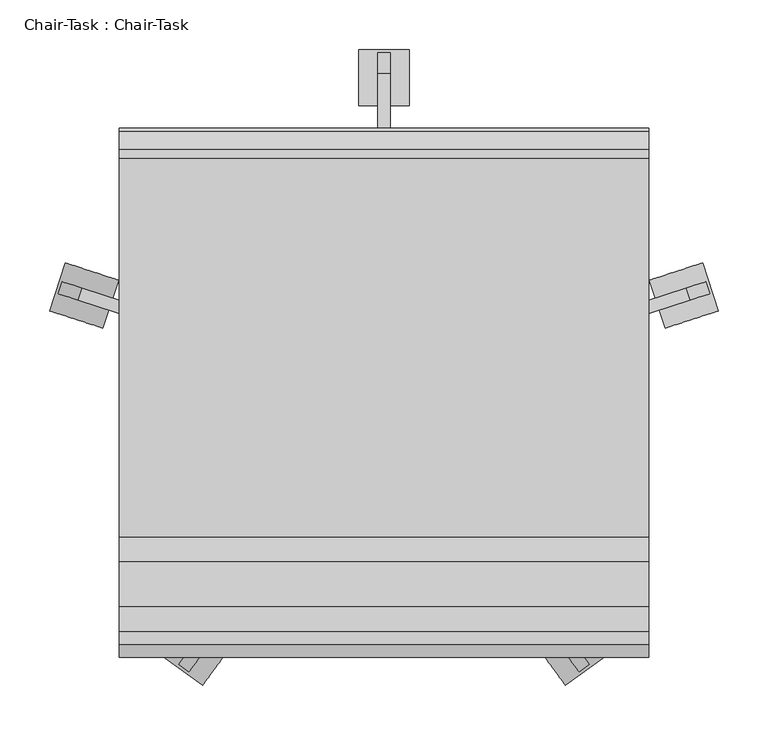
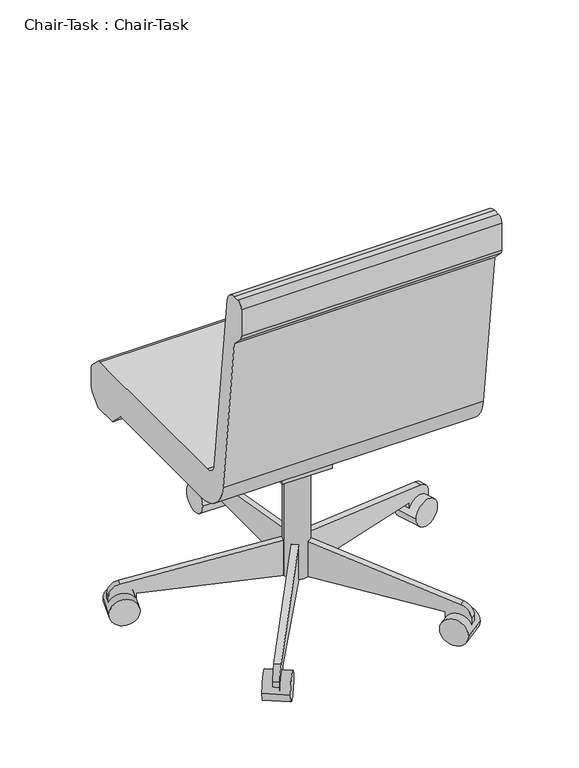
"""IFC4 building model written with IfcOpenShell, lengths in millimetres: furniture geometry, Chair-Task : Chair-Task."""

from ifc_helpers import new_model, si_unit, point, frame, frame_2d, origin, place, context, project, spatial, polyline, circle_curve, trimmed, segment, composite_curve, outline, extrude, source, transform, mapped, element, save


def chair_task_chair_task_b7f3823b(model_context):
    return source(origin(), model_context, "Body", "SweptSolid", [
        extrude(outline(composite_curve([segment(trimmed(circle_curve(frame_2d((140.9908197, 18.9459016)), 25.4), [point((115.5908197, 18.9459016))], [point((166.3908197, 18.9459016))], False, "CARTESIAN"), True, "CONTINUOUS"), segment(trimmed(circle_curve(frame_2d((140.9908197, 18.9459016)), 25.4), [point((166.3908197, 18.9459016))], [point((115.5908197, 18.9459016))], False, "CARTESIAN"), True, "CONTINUOUS")], self_intersect=False)), frame((0.0, 0.0, 53.5835944), z_axis=(0.0, 0.0, 1.0), x_axis=(1.0, 0.0, 0.0)), (0.0, 0.0, 1.0), 330.5914056),
        extrude(outline(composite_curve([segment(trimmed(circle_curve(frame_2d((0.0, -28.2002727)), 28.2002727), [point((0.0, -56.4005455))], [point((0.0, 0.0))], False, "CARTESIAN"), True, "CONTINUOUS"), segment(trimmed(circle_curve(frame_2d((0.0, -28.2002727)), 28.2002727), [point((0.0, 0.0))], [point((0.0, -56.4005455))], False, "CARTESIAN"), True, "CONTINUOUS")], self_intersect=False)), frame((477.6203484, 101.6163254, 28.1835944), z_axis=(-0.3090169943749423, 0.9510565162951553, 0.0), x_axis=(0.0, 0.0, 1.0)), (0.0, 0.0, 1.0), 50.8),
        extrude(outline(composite_curve([segment(polyline([(-25.4, 0.0), (0.0, 0.0), (0.0, -50.8), (-24.303053, -50.8)]), True, "CONTINUOUS"), segment(trimmed(circle_curve(frame_2d((-24.303053, -25.4)), 25.4), [point((-24.303053, -50.8))], [point((-49.3171699, -29.8106637))], False, "CARTESIAN"), True, "CONTINUOUS"), segment(polyline([(-49.3171699, -29.8106637), (-101.6, 266.7), (-101.6, 292.1), (-25.4, 292.1), (-25.4, 0.0)]), True, "CONTINUOUS")], self_intersect=False)), frame((420.756686, 103.1705568, 28.1835944), z_axis=(-0.3090169943749423, 0.9510565162951553, 0.0), x_axis=(0.0, 0.0, -1.0)), (0.0, 0.0, 1.0), 12.7),
        extrude(outline(composite_curve([segment(trimmed(circle_curve(frame_2d((0.0, -28.2002727)), 28.2002727), [point((0.0, -56.4005455))], [point((0.0, 0.0))], False, "CARTESIAN"), True, "CONTINUOUS"), segment(trimmed(circle_curve(frame_2d((0.0, -28.2002727)), 28.2002727), [point((0.0, 0.0))], [point((0.0, -56.4005455))], False, "CARTESIAN"), True, "CONTINUOUS")], self_intersect=False)), frame((323.63931, -275.6612394, 28.1835944), z_axis=(0.8090169943749499, 0.5877852522924699, 0.0), x_axis=(0.0, 0.0, 1.0)), (0.0, 0.0, 1.0), 50.8),
        extrude(outline(composite_curve([segment(polyline([(-25.4, 0.0), (0.0, 0.0), (0.0, -50.8), (-24.303053, -50.8)]), True, "CONTINUOUS"), segment(trimmed(circle_curve(frame_2d((-24.303053, -25.3999999)), 25.4), [point((-24.303053, -50.8))], [point((-49.3171699, -29.8106636))], False, "CARTESIAN"), True, "CONTINUOUS"), segment(polyline([(-49.3171699, -29.8106636), (-101.6, 266.7), (-101.6, 292.1), (-25.4, 292.1), (-25.4, 0.0)]), True, "CONTINUOUS")], self_intersect=False)), frame((307.545634, -221.1003988, 28.1835944), z_axis=(0.8090169943749499, 0.5877852522924699, 0.0), x_axis=(0.0, 0.0, -1.0)), (0.0, 0.0, 1.0), 12.7),
        extrude(outline(composite_curve([segment(trimmed(circle_curve(frame_2d((0.0, -28.2002727)), 28.2002727), [point((0.0, -56.4005455))], [point((0.0, 0.0))], False, "CARTESIAN"), True, "CONTINUOUS"), segment(trimmed(circle_curve(frame_2d((0.0, -28.2002727)), 28.2002727), [point((0.0, 0.0))], [point((0.0, -56.4005455))], False, "CARTESIAN"), True, "CONTINUOUS")], self_intersect=False)), frame((-41.6576707, -275.6612394, 28.1835944), z_axis=(-0.8090169943749458, 0.5877852522924754, 0.0), x_axis=(0.0, 0.0, -1.0)), (0.0, 0.0, 1.0), 50.8),
        extrude(outline(composite_curve([segment(polyline([(25.4, 0.0), (25.4, 292.1), (101.6, 292.1), (101.6, 266.7), (49.3171699, -29.8106637)]), True, "CONTINUOUS"), segment(trimmed(circle_curve(frame_2d((24.303053, -25.3999999)), 25.4), [point((49.3171699, -29.8106637))], [point((24.303053, -50.8))], False, "CARTESIAN"), True, "CONTINUOUS"), segment(polyline([(24.303053, -50.8), (0.0, -50.8), (0.0, 0.0), (25.4, 0.0)]), True, "CONTINUOUS")], self_intersect=False)), frame((-25.5639946, -221.1003988, 28.1835944), z_axis=(-0.8090169943749459, 0.5877852522924754, 0.0), x_axis=(0.0, 0.0, 1.0)), (0.0, 0.0, 1.0), 12.7),
        extrude(outline(composite_curve([segment(trimmed(circle_curve(frame_2d((0.0, -28.2002727)), 28.2002727), [point((0.0, -56.4005454))], [point((0.0, 0.0))], False, "CARTESIAN"), True, "CONTINUOUS"), segment(trimmed(circle_curve(frame_2d((0.0, -28.2002727)), 28.2002727), [point((0.0, 0.0))], [point((0.0, -56.4005454))], False, "CARTESIAN"), True, "CONTINUOUS")], self_intersect=False)), frame((-195.638709, 101.6163254, 28.1835944), z_axis=(0.3090169943749487, 0.9510565162951532, 0.0), x_axis=(0.0, 0.0, -1.0)), (0.0, 0.0, 1.0), 50.8),
        extrude(outline(composite_curve([segment(polyline([(25.4, 0.0), (25.4, 292.1000001), (101.6, 292.1000001), (101.6, 266.7), (49.3171699, -29.8106636)]), True, "CONTINUOUS"), segment(trimmed(circle_curve(frame_2d((24.303053, -25.4)), 25.4), [point((49.3171699, -29.8106636))], [point((24.303053, -50.8))], False, "CARTESIAN"), True, "CONTINUOUS"), segment(polyline([(24.303053, -50.8), (0.0, -50.8), (0.0, 0.0), (25.4, 0.0)]), True, "CONTINUOUS")], self_intersect=False)), frame((-138.7750467, 103.1705568, 28.1835944), z_axis=(0.3090169943749487, 0.9510565162951532, 0.0), x_axis=(0.0, 0.0, 1.0)), (0.0, 0.0, 1.0), 12.7),
        extrude(outline(composite_curve([segment(trimmed(circle_curve(frame_2d((336.4459016, 28.1835944)), 28.2002727), [point((308.2456289, 28.1835944))], [point((364.6461744, 28.1835944))], False, "CARTESIAN"), True, "CONTINUOUS"), segment(trimmed(circle_curve(frame_2d((336.4459016, 28.1835944)), 28.2002727), [point((364.6461744, 28.1835944))], [point((308.2456289, 28.1835944))], False, "CARTESIAN"), True, "CONTINUOUS")], self_intersect=False)), frame((115.5908197, 0.0, 0.0), z_axis=(1.0, 0.0, 0.0), x_axis=(0.0, 1.0, 0.0)), (0.0, 0.0, 1.0), 50.8),
        extrude(outline(composite_curve([segment(polyline([(311.0459016, 53.5835944), (18.9459016, 53.5835944), (18.9459016, 129.7835944), (44.3459016, 129.7835944), (340.8565654, 77.5007643)]), True, "CONTINUOUS"), segment(trimmed(circle_curve(frame_2d((336.4459016, 52.4866474)), 25.4), [point((340.8565654, 77.5007643))], [point((361.8459016, 52.4866474))], False, "CARTESIAN"), True, "CONTINUOUS"), segment(polyline([(361.8459016, 52.4866474), (361.8459016, 28.1835944), (311.0459016, 28.1835944), (311.0459016, 53.5835944)]), True, "CONTINUOUS")], self_intersect=False)), frame((134.6408197, 0.0, 0.0), z_axis=(1.0, 0.0, 0.0), x_axis=(0.0, 1.0, 0.0)), (0.0, 0.0, 1.0), 12.7),
        extrude(outline(polyline([(69.7459016, 383.7835944), (69.7459016, 371.0835944), (18.9459016, 283.0954134), (-19.1540984, 283.0954134), (-19.1540984, 383.7835944), (69.7459016, 383.7835944)])), frame((90.1908197, 0.0, 0.0), z_axis=(1.0, 0.0, 0.0), x_axis=(0.0, 1.0, 0.0)), (0.0, 0.0, 1.0), 101.6),
        extrude(outline(composite_curve([segment(polyline([(-126.2050455, 457.2), (255.0102301, 457.2)]), True, "CONTINUOUS"), segment(trimmed(circle_curve(frame_2d((255.0102301, 444.5)), 12.7), [point((255.0102301, 457.2))], [point((263.9604301, 453.510212))], False, "CARTESIAN"), True, "CONTINUOUS"), segment(polyline([(263.9604301, 453.510212), (281.8961016, 435.6939999)]), True, "CONTINUOUS"), segment(trimmed(circle_curve(frame_2d((272.9459016, 426.6837879)), 12.7), [point((281.8961016, 435.6939999))], [point((285.6459016, 426.6837879))], False, "CARTESIAN"), True, "CONTINUOUS"), segment(polyline([(285.6459016, 426.6837879), (285.6459016, 391.6405184)]), True, "CONTINUOUS"), segment(trimmed(circle_curve(frame_2d((260.2459016, 391.6405184)), 25.4), [point((285.6459016, 391.6405184))], [point((278.2663256, 373.7401184))], False, "CARTESIAN"), True, "CONTINUOUS"), segment(polyline([(278.2663256, 373.7401184), (260.2470284, 355.6), (209.4470284, 355.6), (181.0744602, 383.7835944), (-107.1089978, 383.7835944)]), True, "CONTINUOUS"), segment(trimmed(circle_curve(frame_2d((-107.1089978, 459.9835944)), 76.2), [point((-107.1089978, 383.7835944))], [point((-182.7870738, 451.0802913))], False, "CARTESIAN"), True, "CONTINUOUS"), segment(polyline([(-182.7870738, 451.0802913), (-222.3540984, 787.4), (-244.0343545, 809.0802561)]), True, "CONTINUOUS"), segment(trimmed(circle_curve(frame_2d((-235.0540984, 818.0605122)), 12.7), [point((-244.0343545, 809.0802561))], [point((-247.7540984, 818.0605122))], False, "CARTESIAN"), True, "CONTINUOUS"), segment(polyline([(-247.7540984, 818.0605122), (-247.7540984, 876.3)]), True, "CONTINUOUS"), segment(trimmed(circle_curve(frame_2d((-235.0540984, 876.3)), 12.7), [point((-247.7540984, 876.3))], [point((-235.0540984, 889.0))], False, "CARTESIAN"), True, "CONTINUOUS"), segment(polyline([(-235.0540984, 889.0), (-222.1789239, 889.0)]), True, "CONTINUOUS"), segment(trimmed(circle_curve(frame_2d((-222.1789239, 863.6)), 25.4), [point((-222.1789239, 889.0))], [point((-196.9528985, 866.5677677))], False, "CARTESIAN"), True, "CONTINUOUS"), segment(polyline([(-196.9528985, 866.5677677), (-151.4310708, 479.6322323)]), True, "CONTINUOUS"), segment(trimmed(circle_curve(frame_2d((-126.2050455, 482.6)), 25.4), [point((-151.4310708, 479.6322323))], [point((-126.2050455, 457.2))], True, "CARTESIAN"), True, "CONTINUOUS")], self_intersect=False)), frame((-125.7091803, 0.0, 0.0), z_axis=(1.0, 0.0, 0.0), x_axis=(0.0, 1.0, 0.0)), (0.0, 0.0, 1.0), 533.4),
    ])


if __name__ == "__main__":
    model = new_model("IFC4")
    model_context = context("Model", 3, world=origin())
    ifc_project = project(units=[si_unit("LENGTHUNIT", "METRE", prefix="MILLI")], contexts=[model_context])
    site = spatial("IfcSite", under=ifc_project)
    building = spatial("IfcBuilding", under=site)
    placement = place(None, origin())
    chair_task_chair_task_shape = chair_task_chair_task_b7f3823b(model_context)
    element("IfcFurniture", 1, ObjectType="Chair-Task : Chair-Task", at=placement, inside=building, context=model_context, shape_type="MappedRepresentation", body=[
        mapped(chair_task_chair_task_shape, transform((0.0, 0.0, 0.0), x_axis=(1.0, 0.0, 0.0), y_axis=(0.0, 1.0, 0.0), z_axis=(0.0, 0.0, 1.0))),
    ])
    save(model, "model.ifc")

# Revit data of these elements
# Type "Chair-Task : Chair-Task"
#   Assembly Code = "E2020200"
#   Base Material = Plastic - Black
#   Caster Material = Plastic - Black
#   Seat/Back Material = Textile - Slate Blue
#   Default Elevation = 0
# Element 1 (IfcFurniture, "Chair-Task : Chair-Task")
#   Materials on its faces: "Plastic - Black", "Textile - Slate Blue"
# Materials
#   "Plastic - Black": colour RGB 0 0 0, transparency 0.7
#   "Textile - Slate Blue": class "Fabric", colour RGB 98 102 118, transparency 0
